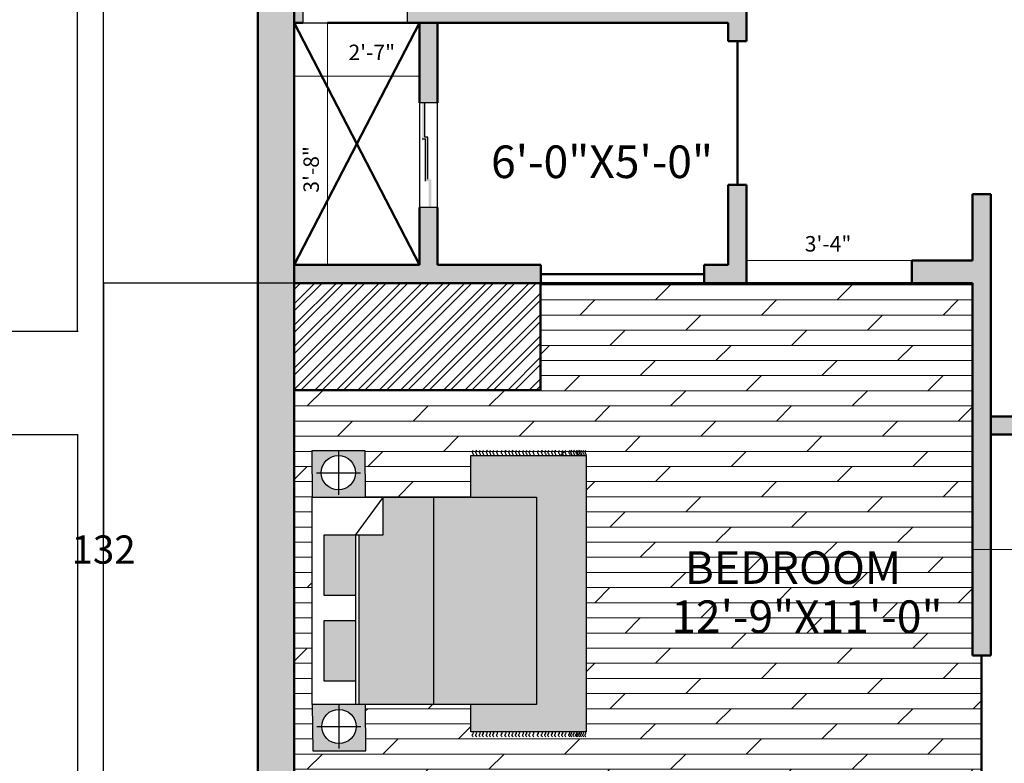
# Model space of a CAD drawing. Units: inches. Extents: x 1381 to 2246, y 1317 to 2168.
# Tile 11 of 15: x 1804 to 2048, y 1591 to 1776. Entities that reach past the tile are written whole.
import ezdxf

# ---------------------------------------------------------------- set-up
doc = ezdxf.new("R2010")
doc.units = ezdxf.units.IN
doc.header["$MEASUREMENT"] = 0
for name, color, linetype, lineweight in [('A-ANNO-DIMS', 2, 'Continuous', 18), ('A-ANNO-TEXT', 7, 'Continuous', 18), ('A-AREA-IDEN', 3, 'Continuous', 25), ('A-FLOR-PATT', 252, 'Continuous', 13), ('A-FURN', 8, 'Continuous', 18), ('A-GLAZ', 4, 'Continuous', 25), ('A-WALL', 7, 'Continuous', 50), ('A-WALL-PATT', 8, 'Continuous', 13)]:
    doc.layers.add(name, color=color, linetype=linetype, lineweight=lineweight)
doc.layers.add('furniture', color=250, linetype='Continuous')
doc.styles.get("Standard").update_dxf_attribs({"font": 'arial.ttf'})
doc.dimstyles.get("Standard").update_dxf_attribs({"dimtxt": 7, "dimasz": 0.18, "dimexe": 0.18, "dimexo": 0.0625, "dimgap": 0.09, "dimtad": 0, "dimtih": 1, "dimtoh": 1, "dimdec": 1, "dimzin": 0, "dimdsep": 46, "dimlunit": 3, "dimtxsty": 'Standard', "dimcen": 0.09, "dimadec": 0, "dimazin": 0, "dimtfac": 1, "dimtdec": 1, "dimtofl": 0, "dimtmove": 0, "dimatfit": 3, "dimfxl": 1, "dimtolj": 1, "dimtzin": 0, "dimarcsym": 0})

# ---------------------------------------------------------------- blocks, each defined once
blk = doc.blocks.new('CARPET')
at = {"layer": 'furniture'}
for p, q in [((-51.53, -98.11), (-51.53, -55.12)), ((-51.53, -55.12), (-41.27, -55.12)), ((36, -55.12), (51.55, -55.12)), ((51.55, -55.12), (51.55, -98.11)), ((51.55, -98.11), (-51.53, -98.11))]:
    blk.add_line(p, q, dxfattribs=at)
for points, knots in [([(-53.37, -55.99), (-53.22, -55.8), (-52.9, -55.41), (-52.34, -55.8), (-51.89, -56.08), (-51.65, -55.91), (-51.53, -55.83)], [0, 0, 0, 0, 0.653278, 1.290138, 1.740457, 2.114451, 2.114451, 2.114451, 2.114451]), ([(-53.37, -57.26), (-53.22, -57.07), (-52.9, -56.67), (-52.34, -57.07), (-51.89, -57.35), (-51.65, -57.17), (-51.53, -57.1)], [0, 0, 0, 0, 0.653278, 1.290138, 1.740457, 2.114451, 2.114451, 2.114451, 2.114451]), ([(-53.37, -58.59), (-53.22, -58.4), (-52.9, -58.01), (-52.34, -58.4), (-51.89, -58.68), (-51.65, -58.5), (-51.53, -58.43)], [0, 0, 0, 0, 0.653278, 1.290138, 1.740457, 2.114451, 2.114451, 2.114451, 2.114451]), ([(53.37, -55.99), (53.22, -55.8), (52.9, -55.41), (52.34, -55.8), (51.89, -56.08), (51.65, -55.91), (51.53, -55.83)], [0, 0, 0, 0, 0.653278, 1.290138, 1.740457, 2.114451, 2.114451, 2.114451, 2.114451]), ([(53.37, -57.26), (53.22, -57.07), (52.9, -56.67), (52.34, -57.07), (51.89, -57.35), (51.65, -57.17), (51.53, -57.1)], [0, 0, 0, 0, 0.653278, 1.290138, 1.740457, 2.114451, 2.114451, 2.114451, 2.114451]), ([(53.37, -58.59), (53.22, -58.4), (52.9, -58.01), (52.34, -58.4), (51.89, -58.68), (51.65, -58.5), (51.53, -58.43)], [0, 0, 0, 0, 0.653278, 1.290138, 1.740457, 2.114451, 2.114451, 2.114451, 2.114451]), ([(-53.37, -59.78), (-53.22, -59.58), (-52.9, -59.19), (-52.34, -59.58), (-51.89, -59.86), (-51.65, -59.69), (-51.53, -59.61)], [0, 0, 0, 0, 0.653278, 1.290138, 1.740457, 2.114451, 2.114451, 2.114451, 2.114451]), ([(-53.37, -61.22), (-53.22, -61.02), (-52.9, -60.63), (-52.34, -61.02), (-51.89, -61.3), (-51.65, -61.13), (-51.53, -61.05)], [0, 0, 0, 0, 0.653278, 1.290138, 1.740457, 2.114451, 2.114451, 2.114451, 2.114451]), ([(-53.37, -62.44), (-53.22, -62.25), (-52.9, -61.86), (-52.34, -62.25), (-51.89, -62.53), (-51.65, -62.36), (-51.53, -62.28)], [0, 0, 0, 0, 0.653278, 1.290138, 1.740457, 2.114451, 2.114451, 2.114451, 2.114451]), ([(53.37, -59.78), (53.22, -59.58), (52.9, -59.19), (52.34, -59.58), (51.89, -59.86), (51.65, -59.69), (51.53, -59.61)], [0, 0, 0, 0, 0.653278, 1.290138, 1.740457, 2.114451, 2.114451, 2.114451, 2.114451]), ([(53.37, -61.22), (53.22, -61.02), (52.9, -60.63), (52.34, -61.02), (51.89, -61.3), (51.65, -61.13), (51.53, -61.05)], [0, 0, 0, 0, 0.653278, 1.290138, 1.740457, 2.114451, 2.114451, 2.114451, 2.114451]), ([(53.37, -62.44), (53.22, -62.25), (52.9, -61.86), (52.34, -62.25), (51.89, -62.53), (51.65, -62.36), (51.53, -62.28)], [0, 0, 0, 0, 0.653278, 1.290138, 1.740457, 2.114451, 2.114451, 2.114451, 2.114451]), ([(-53.37, -63.63), (-53.22, -63.43), (-52.9, -63.04), (-52.34, -63.43), (-51.89, -63.72), (-51.65, -63.54), (-51.53, -63.46)], [0, 0, 0, 0, 0.653278, 1.290138, 1.740457, 2.114451, 2.114451, 2.114451, 2.114451]), ([(-53.37, -65.07), (-53.22, -64.87), (-52.9, -64.48), (-52.34, -64.87), (-51.89, -65.15), (-51.65, -64.98), (-51.53, -64.9)], [0, 0, 0, 0, 0.653278, 1.290138, 1.740457, 2.114451, 2.114451, 2.114451, 2.114451]), ([(53.37, -63.63), (53.22, -63.43), (52.9, -63.04), (52.34, -63.43), (51.89, -63.72), (51.65, -63.54), (51.53, -63.46)], [0, 0, 0, 0, 0.653278, 1.290138, 1.740457, 2.114451, 2.114451, 2.114451, 2.114451]), ([(53.37, -65.07), (53.22, -64.87), (52.9, -64.48), (52.34, -64.87), (51.89, -65.15), (51.65, -64.98), (51.53, -64.9)], [0, 0, 0, 0, 0.653278, 1.290138, 1.740457, 2.114451, 2.114451, 2.114451, 2.114451]), ([(-53.37, -66.76), (-53.22, -66.56), (-52.9, -66.17), (-52.34, -66.56), (-51.89, -66.84), (-51.65, -66.67), (-51.53, -66.59)], [0, 0, 0, 0, 0.653278, 1.290138, 1.740457, 2.114451, 2.114451, 2.114451, 2.114451]), ([(-53.37, -68.2), (-53.22, -68), (-52.9, -67.61), (-52.34, -68), (-51.89, -68.28), (-51.65, -68.11), (-51.53, -68.03)], [0, 0, 0, 0, 0.653278, 1.290138, 1.740457, 2.114451, 2.114451, 2.114451, 2.114451]), ([(-53.37, -69.53), (-53.22, -69.33), (-52.9, -68.94), (-52.34, -69.33), (-51.89, -69.61), (-51.65, -69.44), (-51.53, -69.36)], [0, 0, 0, 0, 0.653278, 1.290138, 1.740457, 2.114451, 2.114451, 2.114451, 2.114451]), ([(53.37, -66.76), (53.22, -66.56), (52.9, -66.17), (52.34, -66.56), (51.89, -66.84), (51.65, -66.67), (51.53, -66.59)], [0, 0, 0, 0, 0.653278, 1.290138, 1.740457, 2.114451, 2.114451, 2.114451, 2.114451]), ([(53.37, -68.2), (53.22, -68), (52.9, -67.61), (52.34, -68), (51.89, -68.28), (51.65, -68.11), (51.53, -68.03)], [0, 0, 0, 0, 0.653278, 1.290138, 1.740457, 2.114451, 2.114451, 2.114451, 2.114451]), ([(53.37, -69.53), (53.22, -69.33), (52.9, -68.94), (52.34, -69.33), (51.89, -69.61), (51.65, -69.44), (51.53, -69.36)], [0, 0, 0, 0, 0.653278, 1.290138, 1.740457, 2.114451, 2.114451, 2.114451, 2.114451]), ([(-53.37, -70.79), (-53.22, -70.6), (-52.9, -70.21), (-52.34, -70.6), (-51.89, -70.88), (-51.65, -70.7), (-51.53, -70.63)], [0, 0, 0, 0, 0.653278, 1.290138, 1.740457, 2.114451, 2.114451, 2.114451, 2.114451]), ([(-53.37, -72.12), (-53.22, -71.93), (-52.9, -71.54), (-52.34, -71.93), (-51.89, -72.21), (-51.65, -72.04), (-51.53, -71.96)], [0, 0, 0, 0, 0.653278, 1.290138, 1.740457, 2.114451, 2.114451, 2.114451, 2.114451]), ([(-53.37, -73.31), (-53.22, -73.11), (-52.9, -72.72), (-52.34, -73.11), (-51.89, -73.4), (-51.65, -73.22), (-51.53, -73.14)], [0, 0, 0, 0, 0.653278, 1.290138, 1.740457, 2.114451, 2.114451, 2.114451, 2.114451]), ([(53.37, -70.79), (53.22, -70.6), (52.9, -70.21), (52.34, -70.6), (51.89, -70.88), (51.65, -70.7), (51.53, -70.63)], [0, 0, 0, 0, 0.653278, 1.290138, 1.740457, 2.114451, 2.114451, 2.114451, 2.114451]), ([(53.37, -72.12), (53.22, -71.93), (52.9, -71.54), (52.34, -71.93), (51.89, -72.21), (51.65, -72.04), (51.53, -71.96)], [0, 0, 0, 0, 0.653278, 1.290138, 1.740457, 2.114451, 2.114451, 2.114451, 2.114451]), ([(53.37, -73.31), (53.22, -73.11), (52.9, -72.72), (52.34, -73.11), (51.89, -73.4), (51.65, -73.22), (51.53, -73.14)], [0, 0, 0, 0, 0.653278, 1.290138, 1.740457, 2.114451, 2.114451, 2.114451, 2.114451]), ([(-53.37, -74.75), (-53.22, -74.55), (-52.9, -74.16), (-52.34, -74.55), (-51.89, -74.83), (-51.65, -74.66), (-51.53, -74.58)], [0, 0, 0, 0, 0.653278, 1.290138, 1.740457, 2.114451, 2.114451, 2.114451, 2.114451]), ([(-53.37, -75.98), (-53.22, -75.78), (-52.9, -75.39), (-52.34, -75.78), (-51.89, -76.06), (-51.65, -75.89), (-51.53, -75.81)], [0, 0, 0, 0, 0.653278, 1.290138, 1.740457, 2.114451, 2.114451, 2.114451, 2.114451]), ([(-53.37, -77.16), (-53.22, -76.96), (-52.9, -76.57), (-52.34, -76.96), (-51.89, -77.25), (-51.65, -77.07), (-51.53, -76.99)], [0, 0, 0, 0, 0.653278, 1.290138, 1.740457, 2.114451, 2.114451, 2.114451, 2.114451]), ([(53.37, -74.75), (53.22, -74.55), (52.9, -74.16), (52.34, -74.55), (51.89, -74.83), (51.65, -74.66), (51.53, -74.58)], [0, 0, 0, 0, 0.653278, 1.290138, 1.740457, 2.114451, 2.114451, 2.114451, 2.114451]), ([(53.37, -75.98), (53.22, -75.78), (52.9, -75.39), (52.34, -75.78), (51.89, -76.06), (51.65, -75.89), (51.53, -75.81)], [0, 0, 0, 0, 0.653278, 1.290138, 1.740457, 2.114451, 2.114451, 2.114451, 2.114451]), ([(53.37, -77.16), (53.22, -76.96), (52.9, -76.57), (52.34, -76.96), (51.89, -77.25), (51.65, -77.07), (51.53, -76.99)], [0, 0, 0, 0, 0.653278, 1.290138, 1.740457, 2.114451, 2.114451, 2.114451, 2.114451]), ([(-53.37, -78.6), (-53.22, -78.4), (-52.9, -78.01), (-52.34, -78.4), (-51.89, -78.68), (-51.65, -78.51), (-51.53, -78.43)], [0, 0, 0, 0, 0.653278, 1.290138, 1.740457, 2.114451, 2.114451, 2.114451, 2.114451]), ([(-53.37, -80.29), (-53.22, -80.09), (-52.9, -79.7), (-52.34, -80.09), (-51.89, -80.37), (-51.65, -80.2), (-51.53, -80.12)], [0, 0, 0, 0, 0.653278, 1.290138, 1.740457, 2.114451, 2.114451, 2.114451, 2.114451]), ([(53.37, -78.6), (53.22, -78.4), (52.9, -78.01), (52.34, -78.4), (51.89, -78.68), (51.65, -78.51), (51.53, -78.43)], [0, 0, 0, 0, 0.653278, 1.290138, 1.740457, 2.114451, 2.114451, 2.114451, 2.114451]), ([(53.37, -80.29), (53.22, -80.09), (52.9, -79.7), (52.34, -80.09), (51.89, -80.37), (51.65, -80.2), (51.53, -80.12)], [0, 0, 0, 0, 0.653278, 1.290138, 1.740457, 2.114451, 2.114451, 2.114451, 2.114451]), ([(-53.37, -81.73), (-53.22, -81.53), (-52.9, -81.14), (-52.34, -81.53), (-51.89, -81.81), (-51.65, -81.64), (-51.53, -81.56)], [0, 0, 0, 0, 0.653278, 1.290138, 1.740457, 2.114451, 2.114451, 2.114451, 2.114451]), ([(-53.37, -83.06), (-53.22, -82.86), (-52.9, -82.47), (-52.34, -82.86), (-51.89, -83.14), (-51.65, -82.97), (-51.53, -82.89)], [0, 0, 0, 0, 0.653278, 1.290138, 1.740457, 2.114451, 2.114451, 2.114451, 2.114451]), ([(-53.37, -84.18), (-53.22, -83.99), (-52.9, -83.6), (-52.34, -83.99), (-51.89, -84.27), (-51.65, -84.09), (-51.53, -84.02)], [0, 0, 0, 0, 0.653278, 1.290138, 1.740457, 2.114451, 2.114451, 2.114451, 2.114451]), ([(53.37, -81.73), (53.22, -81.53), (52.9, -81.14), (52.34, -81.53), (51.89, -81.81), (51.65, -81.64), (51.53, -81.56)], [0, 0, 0, 0, 0.653278, 1.290138, 1.740457, 2.114451, 2.114451, 2.114451, 2.114451]), ([(53.37, -83.06), (53.22, -82.86), (52.9, -82.47), (52.34, -82.86), (51.89, -83.14), (51.65, -82.97), (51.53, -82.89)], [0, 0, 0, 0, 0.653278, 1.290138, 1.740457, 2.114451, 2.114451, 2.114451, 2.114451]), ([(53.37, -84.18), (53.22, -83.99), (52.9, -83.6), (52.34, -83.99), (51.89, -84.27), (51.65, -84.09), (51.53, -84.02)], [0, 0, 0, 0, 0.653278, 1.290138, 1.740457, 2.114451, 2.114451, 2.114451, 2.114451]), ([(-53.37, -85.51), (-53.22, -85.32), (-52.9, -84.93), (-52.34, -85.32), (-51.89, -85.6), (-51.65, -85.42), (-51.53, -85.35)], [0, 0, 0, 0, 0.653278, 1.290138, 1.740457, 2.114451, 2.114451, 2.114451, 2.114451]), ([(-53.37, -86.7), (-53.22, -86.5), (-52.9, -86.11), (-52.34, -86.5), (-51.89, -86.78), (-51.65, -86.61), (-51.53, -86.53)], [0, 0, 0, 0, 0.653278, 1.290138, 1.740457, 2.114451, 2.114451, 2.114451, 2.114451]), ([(-53.37, -88.14), (-53.22, -87.94), (-52.9, -87.55), (-52.34, -87.94), (-51.89, -88.22), (-51.65, -88.05), (-51.53, -87.97)], [0, 0, 0, 0, 0.653278, 1.290138, 1.740457, 2.114451, 2.114451, 2.114451, 2.114451]), ([(53.37, -85.51), (53.22, -85.32), (52.9, -84.93), (52.34, -85.32), (51.89, -85.6), (51.65, -85.42), (51.53, -85.35)], [0, 0, 0, 0, 0.653278, 1.290138, 1.740457, 2.114451, 2.114451, 2.114451, 2.114451]), ([(53.37, -86.7), (53.22, -86.5), (52.9, -86.11), (52.34, -86.5), (51.89, -86.78), (51.65, -86.61), (51.53, -86.53)], [0, 0, 0, 0, 0.653278, 1.290138, 1.740457, 2.114451, 2.114451, 2.114451, 2.114451]), ([(53.37, -88.14), (53.22, -87.94), (52.9, -87.55), (52.34, -87.94), (51.89, -88.22), (51.65, -88.05), (51.53, -87.97)], [0, 0, 0, 0, 0.653278, 1.290138, 1.740457, 2.114451, 2.114451, 2.114451, 2.114451]), ([(-53.37, -89.36), (-53.22, -89.17), (-52.9, -88.78), (-52.34, -89.17), (-51.89, -89.45), (-51.65, -89.28), (-51.53, -89.2)], [0, 0, 0, 0, 0.653278, 1.290138, 1.740457, 2.114451, 2.114451, 2.114451, 2.114451]), ([(-53.37, -90.55), (-53.22, -90.35), (-52.9, -89.96), (-52.34, -90.35), (-51.89, -90.64), (-51.65, -90.46), (-51.53, -90.38)], [0, 0, 0, 0, 0.653278, 1.290138, 1.740457, 2.114451, 2.114451, 2.114451, 2.114451]), ([(-53.37, -91.99), (-53.22, -91.79), (-52.9, -91.4), (-52.34, -91.79), (-51.89, -92.07), (-51.65, -91.9), (-51.53, -91.82)], [0, 0, 0, 0, 0.653278, 1.290138, 1.740457, 2.114451, 2.114451, 2.114451, 2.114451]), ([(53.37, -89.36), (53.22, -89.17), (52.9, -88.78), (52.34, -89.17), (51.89, -89.45), (51.65, -89.28), (51.53, -89.2)], [0, 0, 0, 0, 0.653278, 1.290138, 1.740457, 2.114451, 2.114451, 2.114451, 2.114451]), ([(53.37, -90.55), (53.22, -90.35), (52.9, -89.96), (52.34, -90.35), (51.9, -90.63), (51.66, -90.47), (51.55, -90.4)], [0, 0, 0, 0, 0.653278, 1.290138, 1.740457, 2.0926, 2.0926, 2.0926, 2.0926]), ([(53.37, -91.99), (53.22, -91.79), (52.9, -91.4), (52.34, -91.79), (51.9, -92.07), (51.66, -91.91), (51.55, -91.83)], [0, 0, 0, 0, 0.653278, 1.290138, 1.740457, 2.0926, 2.0926, 2.0926, 2.0926]), ([(-53.37, -92.69), (-53.22, -92.48), (-52.9, -92.08), (-52.35, -92.49), (-51.89, -92.77), (-51.65, -92.6), (-51.53, -92.52)], [0, 0, 0, 0, 0.663904, 1.307406, 1.757725, 2.131719, 2.131719, 2.131719, 2.131719]), ([(-53.37, -93.61), (-53.22, -93.42), (-52.9, -93.03), (-52.34, -93.42), (-51.89, -93.7), (-51.65, -93.52), (-51.53, -93.45)], [0, 0, 0, 0, 0.653278, 1.290138, 1.740457, 2.114451, 2.114451, 2.114451, 2.114451]), ([(-53.37, -94.55), (-53.22, -94.35), (-52.9, -93.96), (-52.34, -94.35), (-51.89, -94.63), (-51.65, -94.46), (-51.53, -94.38)], [0, 0, 0, 0, 0.653278, 1.290138, 1.740457, 2.114451, 2.114451, 2.114451, 2.114451]), ([(-53.37, -95.05), (-53.22, -94.85), (-52.9, -94.46), (-52.34, -94.85), (-51.89, -95.14), (-51.65, -94.96), (-51.53, -94.88)], [0, 0, 0, 0, 0.653278, 1.290138, 1.740457, 2.114451, 2.114451, 2.114451, 2.114451]), ([(-53.37, -95.73), (-53.22, -95.54), (-52.9, -95.15), (-52.34, -95.54), (-51.89, -95.82), (-51.65, -95.65), (-51.53, -95.57)], [0, 0, 0, 0, 0.653278, 1.290138, 1.740457, 2.114451, 2.114451, 2.114451, 2.114451]), ([(53.37, -95.78), (53.22, -95.58), (52.9, -95.19), (52.34, -95.58), (51.89, -95.86), (51.65, -95.69), (51.53, -95.61)], [0, 0, 0, 0, 0.653278, 1.290138, 1.740457, 2.114451, 2.114451, 2.114451, 2.114451]), ([(53.37, -92.69), (53.22, -92.49), (52.9, -92.09), (52.34, -92.49), (51.9, -92.77), (51.66, -92.61), (51.55, -92.53)], [0, 0, 0, 0, 0.656792, 1.295826, 1.746145, 2.098292, 2.098292, 2.098292, 2.098292]), ([(53.37, -93.66), (53.22, -93.46), (52.9, -93.07), (52.34, -93.46), (51.9, -93.74), (51.66, -93.58), (51.55, -93.5)], [0, 0, 0, 0, 0.653278, 1.290138, 1.740457, 2.0926, 2.0926, 2.0926, 2.0926]), ([(53.37, -94.59), (53.22, -94.4), (52.9, -94.01), (52.34, -94.4), (51.9, -94.68), (51.66, -94.51), (51.55, -94.44)], [0, 0, 0, 0, 0.653278, 1.290138, 1.740457, 2.0926, 2.0926, 2.0926, 2.0926]), ([(53.37, -95.1), (53.22, -94.9), (52.9, -94.51), (52.34, -94.9), (51.9, -95.18), (51.66, -95.02), (51.55, -94.94)], [0, 0, 0, 0, 0.653278, 1.290138, 1.740457, 2.0926, 2.0926, 2.0926, 2.0926]), ([(-53.37, -96.38), (-53.22, -96.18), (-52.9, -95.79), (-52.34, -96.18), (-51.89, -96.47), (-51.65, -96.29), (-51.53, -96.21)], [0, 0, 0, 0, 0.653278, 1.290138, 1.740457, 2.114451, 2.114451, 2.114451, 2.114451]), ([(-53.37, -97.17), (-53.22, -96.98), (-52.9, -96.59), (-52.34, -96.98), (-51.89, -97.26), (-51.65, -97.08), (-51.53, -97.01)], [0, 0, 0, 0, 0.653278, 1.290138, 1.740457, 2.114451, 2.114451, 2.114451, 2.114451]), ([(-53.37, -97.99), (-53.22, -97.79), (-52.9, -97.4), (-52.34, -97.79), (-51.89, -98.08), (-51.65, -97.9), (-51.53, -97.82)], [0, 0, 0, 0, 0.653278, 1.290138, 1.740457, 2.114451, 2.114451, 2.114451, 2.114451]), ([(53.37, -96.43), (53.22, -96.23), (52.9, -95.84), (52.34, -96.23), (51.89, -96.51), (51.65, -96.34), (51.53, -96.26)], [0, 0, 0, 0, 0.653278, 1.290138, 1.740457, 2.114451, 2.114451, 2.114451, 2.114451]), ([(53.37, -97.22), (53.22, -97.02), (52.9, -96.63), (52.34, -97.02), (51.89, -97.3), (51.65, -97.13), (51.53, -97.05)], [0, 0, 0, 0, 0.653278, 1.290138, 1.740457, 2.114451, 2.114451, 2.114451, 2.114451]), ([(53.37, -97.99), (53.22, -97.79), (52.9, -97.4), (52.34, -97.79), (51.89, -98.08), (51.65, -97.9), (51.53, -97.82)], [0, 0, 0, 0, 0.653278, 1.290138, 1.740457, 2.114451, 2.114451, 2.114451, 2.114451])]:
    blk.add_open_spline(points, degree=3, knots=knots, dxfattribs=at)
blk = doc.blocks.new('A$C58D270C6')
at = {"layer": 'furniture'}
for p, q in [((9.09, 124.13), (9.09, 108.87)), ((1.46, 116.5), (16.73, 116.5)), ((14.97, 94.84), (24.62, 107.92)), ((24.62, 94.93), (24.62, 107.92)), ((42.08, 108), (42.08, 36)), ((14.97, 94.93), (24.62, 94.93)), ((14.97, 94.84), (14.97, 36)), ((16.22, 94.93), (16.22, 36)), ((9.25, 36), (9.25, 20.74)), ((1.62, 28.37), (16.88, 28.37))]:
    blk.add_line(p, q, dxfattribs=at)
for points in [[(18.5, 108), (18.34, 124.13), (-0.16, 124.13), (0, 108)], [(0, 108), (77.91, 108), (77.91, 36), (0, 36)], [(4.09, 94.93), (14.97, 94.93), (14.97, 73.83), (4.09, 73.83)], [(4.09, 65.23), (14.97, 65.23), (14.97, 44.13), (4.09, 44.13)], [(18.65, 19.87), (18.5, 36), (0, 36), (0.16, 19.87)]]:
    blk.add_lwpolyline(points, close=True, dxfattribs=at)
for centre in [(9.09, 116.5), (9.25, 28.37)]:
    blk.add_circle(centre, 5.95, dxfattribs=at)
at = {"layer": 'furniture', "xscale": 0.9312884925094044, "yscale": 0.9312884925094044, "zscale": 0.9312884925094044, "rotation": 90}
blk.add_blockref('CARPET', (3.79, 74.47), dxfattribs=at)
blk = doc.blocks.new('*D60')
at = {"layer": 'A-ANNO-DIMS', "color": 0, "lineweight": -2, "transparency": 16777216}
for p, q in [((1737.61, 1672.92), (1818.27, 1672.92)), ((1818.09, 1672.74), (1818.09, 1576.08)), ((1818.09, 1472.1), (1818.09, 1568.75)), ((1737.61, 1471.92), (1818.27, 1471.92))]:
    blk.add_line(p, q, dxfattribs=at)
at = {"layer": 'A-ANNO-DIMS', "color": 0, "transparency": 16777216}
for points in [[(1818.06, 1672.74), (1818.12, 1672.74), (1818.09, 1672.92)], [(1818.06, 1472.1), (1818.12, 1472.1), (1818.09, 1471.92)]]:
    blk.add_solid(points, dxfattribs=at)
at = {"layer": 'Defpoints', "color": 0, "transparency": 16777216}
for p in [(1737.55, 1672.92), (1818.09, 1672.92), (1737.55, 1471.92)]:
    blk.add_point(p, dxfattribs=at)
at = {"layer": 'A-ANNO-DIMS', "color": 0, "transparency": 16777216, "insert": (1818.09, 1572.42), "char_height": 7, "attachment_point": 5}
blk.add_mtext('\\A1;201', dxfattribs=at)
blk = doc.blocks.new('*D61')
at = {"layer": 'A-ANNO-DIMS', "color": 0, "lineweight": -2, "transparency": 16777216}
for p, q in [((1737.61, 1911.42), (1818.27, 1911.42)), ((1818.09, 1911.24), (1818.09, 1808.63)), ((1818.09, 1698.7), (1818.09, 1801.3)), ((1737.61, 1698.52), (1818.27, 1698.52))]:
    blk.add_line(p, q, dxfattribs=at)
at = {"layer": 'A-ANNO-DIMS', "color": 0, "transparency": 16777216}
for points in [[(1818.06, 1911.24), (1818.12, 1911.24), (1818.09, 1911.42)], [(1818.06, 1698.7), (1818.12, 1698.7), (1818.09, 1698.52)]]:
    blk.add_solid(points, dxfattribs=at)
at = {"layer": 'Defpoints', "color": 0, "transparency": 16777216}
for p in [(1737.55, 1911.42), (1818.09, 1911.42), (1737.55, 1698.52)]:
    blk.add_point(p, dxfattribs=at)
at = {"layer": 'A-ANNO-DIMS', "color": 0, "transparency": 16777216, "insert": (1818.09, 1804.97), "char_height": 7, "attachment_point": 5}
blk.add_mtext('\\A1;212.9', dxfattribs=at)
blk = doc.blocks.new('*D76')
at = {"layer": 'A-ANNO-DIMS', "color": 0, "lineweight": -2, "transparency": 16777216}
for p, q in [((1862.74, 2092.92), (1824.38, 2092.92)), ((1824.56, 2092.74), (1824.56, 1786.08)), ((1824.56, 1472.1), (1824.56, 1778.75)), ((1862.74, 1471.92), (1824.38, 1471.92))]:
    blk.add_line(p, q, dxfattribs=at)
at = {"layer": 'A-ANNO-DIMS', "color": 0, "transparency": 16777216}
for points in [[(1824.53, 2092.74), (1824.59, 2092.74), (1824.56, 2092.92)], [(1824.53, 1472.1), (1824.59, 1472.1), (1824.56, 1471.92)]]:
    blk.add_solid(points, dxfattribs=at)
at = {"layer": 'Defpoints', "color": 0, "transparency": 16777216}
for p in [(1824.56, 2092.92), (1862.81, 2092.92), (1862.81, 1471.92)]:
    blk.add_point(p, dxfattribs=at)
at = {"layer": 'A-ANNO-DIMS', "color": 0, "transparency": 16777216, "insert": (1824.56, 1782.42), "char_height": 7, "attachment_point": 5}
blk.add_mtext('\\A1;621', dxfattribs=at)
blk = doc.blocks.new('*D81')
at = {"layer": 'A-ANNO-DIMS', "color": 0, "lineweight": -2, "transparency": 16777216}
for p, q in [((1871.74, 1710.42), (1824.38, 1710.42)), ((1824.56, 1710.24), (1824.56, 1648.08)), ((1824.56, 1578.6), (1824.56, 1640.75)), ((1871.74, 1578.42), (1824.38, 1578.42))]:
    blk.add_line(p, q, dxfattribs=at)
at = {"layer": 'A-ANNO-DIMS', "color": 0, "transparency": 16777216}
for points in [[(1824.53, 1710.24), (1824.59, 1710.24), (1824.56, 1710.42)], [(1824.53, 1578.6), (1824.59, 1578.6), (1824.56, 1578.42)]]:
    blk.add_solid(points, dxfattribs=at)
at = {"layer": 'Defpoints', "color": 0, "transparency": 16777216}
for p in [(1824.56, 1710.42), (1871.81, 1710.42), (1871.81, 1578.42)]:
    blk.add_point(p, dxfattribs=at)
at = {"layer": 'A-ANNO-DIMS', "color": 0, "transparency": 16777216, "insert": (1824.56, 1644.42), "char_height": 7, "attachment_point": 5}
blk.add_mtext('\\A1;132', dxfattribs=at)

msp = doc.modelspace()

# ---------------------------------------------------------------- hatches: boundary and pattern name
at = {"layer": 'A-FLOR-PATT'}
h = msp.add_hatch(dxfattribs=at)
h.set_pattern_fill('ANSI32', color=256, scale=10)
h.set_pattern_definition([(45, (415.7542, 0), (-2.6516504, 2.6516504), []), (45, (417.522, 0), (-2.6516504, 2.6516504), [])])
h.paths.add_polyline_path([(1932.8736, 1710.4163), (1871.8052, 1710.4163), (1871.8052, 1683.9148), (1932.8736, 1683.9148)])
h = msp.add_hatch(dxfattribs=at)
h.set_pattern_fill('DOLMIT', color=256, scale=15)
h.paths.add_polyline_path([(2039.8052, 1710.4163), (2024.8052, 1710.4163), (1932.7523, 1710.4163), (1932.7523, 1683.9148), (1871.8052, 1683.9148), (1871.8052, 1578.4163), (2039.8052, 1578.4163), (2039.8052, 1581.7679), (2042.0552, 1581.7679), (2042.0552, 1618.2205), (2039.8052, 1618.2205)])
edge = h.paths.add_edge_path(flags=16)
edge.add_spline(control_points=[(1941.6512, 1599.2474), (1941.7034, 1599.1739), (1941.8185, 1599.0119), (1941.6311, 1598.7103), (1941.372, 1598.3387), (1941.6312, 1598.1308), (1941.7624, 1598.0254)], knot_values=[0, 0, 0, 0, 0.37399428, 0.82431366, 1.46117297, 2.11445126, 2.11445126, 2.11445126, 2.11445126], degree=3, periodic=0)
edge.add_spline(control_points=[(1941.9859, 1599.2474), (1942.0381, 1599.1739), (1942.1532, 1599.0119), (1941.9659, 1598.7103), (1941.7067, 1598.3387), (1941.9659, 1598.1308), (1942.0971, 1598.0254)], knot_values=[0, 0, 0, 0, 0.37399428, 0.82431366, 1.46117297, 2.11445126, 2.11445126, 2.11445126, 2.11445126], degree=3, periodic=0)
edge = h.paths.add_edge_path(flags=16)
edge.add_line((1944.1282, 1667.7293), (1944.1282, 1599.2474))
edge.add_line((1944.1282, 1599.2474), (1915.5728, 1599.2474))
edge.add_line((1915.5728, 1599.2474), (1915.5728, 1606.0382))
edge.add_line((1915.5728, 1606.0382), (1889.4451, 1606.0382))
edge.add_line((1889.4451, 1606.0382), (1889.5561, 1594.5315))
edge.add_line((1889.5561, 1594.5315), (1876.3603, 1594.5315))
edge.add_line((1876.3603, 1594.5315), (1876.2493, 1606.0382))
edge.add_line((1876.2493, 1606.0382), (1876.2493, 1657.3975))
edge.add_line((1876.2493, 1657.3975), (1876.1383, 1668.9042))
edge.add_line((1876.1383, 1668.9042), (1889.3342, 1668.9042))
edge.add_line((1889.3342, 1668.9042), (1889.4451, 1657.3975))
edge.add_line((1889.4451, 1657.3975), (1915.5728, 1657.3975))
edge.add_line((1915.5728, 1657.3975), (1915.5728, 1667.7293))
edge.add_line((1915.5728, 1667.7293), (1941.69, 1667.7293))
edge.add_spline(control_points=[(1941.69, 1667.7293), (1941.7379, 1667.7989), (1941.8471, 1667.9576), (1941.661, 1668.2542), (1941.4024, 1668.626), (1941.6615, 1668.8339), (1941.7927, 1668.9392)], knot_values=[0, 0, 0, 0, 0.3521435, 0.80246288, 1.43932219, 2.09260048, 2.09260048, 2.09260048, 2.09260048], degree=3, periodic=0)
edge.add_spline(control_points=[(1942.1275, 1668.9392), (1941.9963, 1668.8339), (1941.7372, 1668.626), (1941.9957, 1668.2542), (1942.1818, 1667.9576), (1942.0727, 1667.7989), (1942.0248, 1667.7293)], knot_values=[0, 0, 0, 0, 0.65327829, 1.2901376, 1.74045698, 2.09260048, 2.09260048, 2.09260048, 2.09260048], degree=3, periodic=0)
edge.add_line((1942.0248, 1667.7293), (1944.1282, 1667.7293))
h.paths.add_polyline_path([(1893.809, 1657.3422), (1893.809, 1648.0757), (1886.9767, 1648.0757), (1886.9307, 1648.0133), (1886.9307, 1611.8376), (1879.1699, 1611.8376), (1879.1699, 1626.8866), (1886.9307, 1626.8866), (1886.9307, 1633.0267), (1879.1699, 1633.0267), (1879.1699, 1648.0757), (1886.9767, 1648.0757)], flags=0)
h.paths.add_polyline_path([(1886.984, 1663.4608, -1), (1878.4885, 1663.4608, -1)], flags=0)
h.paths.add_polyline_path([(1887.0949, 1600.5947, -1), (1878.5995, 1600.5947, -1)], flags=0)
h.paths.add_polyline_path([(1963.1209, 1621.5603), (2032.2362, 1621.5603), (2032.2362, 1633.9282), (1963.1209, 1633.9282)], flags=24)
h.paths.add_polyline_path([(1966.4202, 1633.6986), (2028.882, 1633.6986), (2028.882, 1646.2317), (1966.4202, 1646.2317)], flags=24)
at = {"layer": 'A-FURN'}
h = msp.add_hatch(color=256, dxfattribs=at)
h.dxf.hatch_style = 1
h.paths.add_polyline_path([(1944.1282, 1667.7293), (1915.5728, 1667.7293), (1915.5728, 1657.3975), (1931.8208, 1657.3975), (1931.8208, 1606.0382), (1915.5728, 1606.0382), (1915.5728, 1599.2474), (1944.1282, 1599.2474)])
h.paths.add_polyline_path([(1882.8472, 1606.0382), (1876.2493, 1606.0382), (1876.3603, 1594.5315), (1889.5561, 1594.5315), (1889.4451, 1606.0382), (1882.8472, 1606.0382), (1882.8472, 1604.8424, -0.41421356), (1887.0949, 1600.5947, -1), (1878.5995, 1600.5947, -0.41421356), (1882.8472, 1604.8424)])
h.paths.add_polyline_path([(1889.3342, 1668.9042), (1882.7362, 1668.9042), (1882.7362, 1667.7085, -0.41421356), (1886.984, 1663.4608, -1), (1878.4885, 1663.4608, -0.41421356), (1882.7362, 1667.7085), (1882.7362, 1668.9042), (1876.1383, 1668.9042), (1876.2493, 1657.3975), (1889.4451, 1657.3975)])
h = msp.add_hatch(color=256, dxfattribs=at)
h.dxf.hatch_style = 1
h.paths.add_polyline_path([(1906.2646, 1657.3975), (1893.8498, 1657.3975), (1893.809, 1657.3422), (1893.809, 1648.0757), (1887.8171, 1648.0757), (1887.8171, 1606.0382), (1906.2646, 1606.0382)])
h.paths.add_polyline_path([(1931.8208, 1657.3975), (1906.2646, 1657.3975), (1906.2646, 1606.0382), (1931.8208, 1606.0382)])
h = msp.add_hatch(color=256, dxfattribs=at)
h.dxf.hatch_style = 1
h.paths.add_polyline_path([(1886.9307, 1626.8866), (1879.1699, 1626.8866), (1879.1699, 1611.8376), (1886.9307, 1611.8376)])
h.paths.add_polyline_path([(1886.9307, 1648.0757), (1879.1699, 1648.0757), (1879.1699, 1633.0267), (1886.9307, 1633.0267)])
at = {"layer": 'A-GLAZ'}
h = msp.add_hatch(color=256, dxfattribs=at)
h.dxf.hatch_style = 1
h.paths.add_polyline_path([(1904.8793, 1736.1591), (1904.8793, 1746.5538), (1904.1533, 1746.5538), (1904.1533, 1755.1129), (1903.4932, 1755.1129), (1903.4932, 1746.1133), (1904.2633, 1746.1133), (1904.2633, 1735.6746), (1905.0552, 1735.6746), (1905.0552, 1729.193), (1905.7814, 1729.193), (1905.7814, 1736.1591)])
at = {"layer": 'A-WALL-PATT'}
h = msp.add_hatch(color=256, dxfattribs=at)
h.dxf.hatch_style = 1
h.paths.add_polyline_path([(1990.4785, 1915.9163), (1929.807, 1915.9163), (1929.807, 1911.4163), (1990.4785, 1911.4163)], flags=17)
h.paths.add_polyline_path([(1900.7902, 1915.9163), (1871.8052, 1915.9163), (1871.8052, 1911.4163), (1900.7902, 1911.4163)], flags=17)
h.paths.add_polyline_path([(2043.2216, 1915.9163), (2038.3052, 1915.9163), (2038.3052, 2035.4163), (2098.0373, 2035.4163), (2098.0373, 2039.9163), (2033.8052, 2039.9163), (2033.8052, 1915.9163), (2028.7731, 1915.9163), (2028.7731, 1911.4163), (2043.2216, 1911.4163)], flags=17)
h.paths.add_polyline_path([(2153.3052, 1915.9163), (2085.2216, 1915.9163), (2085.2216, 1911.4163), (2153.3052, 1911.4163)], flags=17)
h.paths.add_polyline_path([(1935.508, 1911.4163), (1931.008, 1911.4163), (1931.008, 1779.4163), (1899.8394, 1779.4163), (1899.8394, 1774.9163), (1902.8052, 1774.9163), (1979.3052, 1774.9163), (1979.3052, 1770.3401), (1983.8052, 1770.3401), (1983.8052, 1779.4163), (1935.508, 1779.4163)], flags=17)
h.paths.add_polyline_path([(1871.8052, 2083.9163), (2153.3052, 2083.9163), (2153.3052, 2039.9163), (2141.7178, 2039.9163), (2141.7178, 2035.4163), (2153.3052, 2035.4163), (2153.3052, 1471.9163), (2162.3052, 1471.9163), (2162.3052, 2092.9163), (1862.8052, 2092.9163), (1862.8052, 1471.9163), (1904.4174, 1471.9163), (1904.4174, 1480.9163), (1871.8052, 1480.9163), (1871.8052, 1569.4163), (1964.2348, 1569.4163), (1964.2348, 1578.4163), (1871.8052, 1578.4163)])
h.paths.add_polyline_path([(1907.3052, 1729.193), (1902.8052, 1729.193), (1902.8052, 1714.9163), (1871.8052, 1714.9163), (1871.8052, 1710.4163), (1932.8736, 1710.4163), (1932.8736, 1714.9163), (1907.3052, 1714.9163)], flags=17)
h.paths.add_polyline_path([(2044.3052, 1644.4163), (2039.8052, 1644.4163), (2039.8052, 1618.2205), (2044.3052, 1618.2205)], flags=17)
h.paths.add_polyline_path([(2044.3052, 1581.7679), (2039.8052, 1581.7679), (2039.8052, 1578.4163), (2027.577, 1578.4163), (2027.577, 1569.4163), (2044.3052, 1569.4163)], flags=17)
h = msp.add_hatch(color=256, dxfattribs=at)
h.dxf.hatch_style = 1
h.paths.add_polyline_path([(1873.9195, 1779.4163), (1871.8052, 1779.4163), (1871.8052, 1774.9163), (1873.9195, 1774.9163)])
h.paths.add_polyline_path([(1983.8052, 1779.4163), (1935.508, 1779.4163), (1935.508, 1911.4163), (1931.008, 1911.4163), (1931.008, 1779.4163), (1899.8394, 1779.4163), (1899.8394, 1774.9163), (1902.8052, 1774.9163), (1979.3052, 1774.9163), (1979.3052, 1770.3401), (1983.8052, 1770.3401)])
h.paths.add_polyline_path([(1907.3052, 1774.9163), (1902.8052, 1774.9163), (1902.8052, 1755.1129), (1907.3052, 1755.1129)])
h.paths.add_polyline_path([(1983.8052, 1734.7997), (1979.3052, 1734.7997), (1979.3052, 1714.9163), (1973.3503, 1714.9163), (1973.3503, 1710.4163), (1983.8052, 1710.4163)])
h.paths.add_polyline_path([(2044.3052, 1732.454), (2039.8052, 1732.454), (2039.8052, 1716.0149), (2024.8052, 1716.0149), (2024.8052, 1710.4163), (2039.8052, 1710.4163), (2039.8052, 1644.4163), (2044.3052, 1644.4163)])
h.paths.add_polyline_path([(2056.2659, 1677.4163), (2044.3052, 1677.4163), (2044.3052, 1672.9163), (2056.2659, 1672.9163)])
h.paths.add_polyline_path([(2119.6192, 1677.4163), (2104.2659, 1677.4163), (2104.2659, 1672.9163), (2119.6192, 1672.9163)])
h.paths.add_polyline_path([(2012.5552, 1480.9163), (1952.401, 1480.9163), (1952.401, 1471.9163), (2012.5552, 1471.9163)])
h.paths.add_polyline_path([(1870.8149, 1834.6368), (1933.6567, 1834.6368), (1933.6567, 1847.0047), (1870.8149, 1847.0047)], flags=9)

# ---------------------------------------------------------------- linework, layer by layer
at = {"layer": 'A-ANNO-DIMS'}
for p, q in [((1880.034, 1714.9163), (1880.034, 1774.9163)), ((1871.8052, 1761.653), (1902.8052, 1761.653)), ((1983.8052, 1716.0149), (2024.8052, 1716.0149)), ((2039.8052, 1644.4163), (2153.3052, 1644.4163))]:
    msp.add_line(p, q, dxfattribs=at)
at = {"layer": 'A-GLAZ'}
for p, q in [((1873.9195, 1779.4163), (1873.9195, 1774.9163)), ((1899.8394, 1774.9163), (1899.8394, 1779.4163)), ((1873.9195, 1774.9163), (1902.8052, 1774.9163)), ((1907.3052, 1755.1129), (1902.8052, 1755.1129)), ((1902.8052, 1755.1129), (1902.8052, 1729.193)), ((1904.1533, 1746.5538), (1904.1533, 1755.1129)), ((1907.3052, 1729.193), (1907.3052, 1755.1129)), ((1904.8793, 1746.5538), (1904.1533, 1746.5538)), ((1904.8793, 1736.1591), (1904.8793, 1746.5538)), ((1904.2633, 1746.1133), (1903.4932, 1746.1133)), ((1904.2633, 1735.6746), (1904.2633, 1746.1133)), ((1907.3052, 1729.193), (1902.8052, 1729.193))]:
    msp.add_line(p, q, dxfattribs=at)
at = {"layer": 'A-WALL'}
for p, q in [((1862.8052, 2092.9163), (1862.8052, 1471.9163)), ((1871.8052, 2083.9163), (1871.8052, 1578.4163)), ((1983.8052, 1779.4163), (1983.8052, 1770.3401)), ((1902.8052, 1714.9163), (1871.8052, 1774.9163)), ((1871.8052, 1714.9163), (1902.8052, 1774.9163)), ((1871.8052, 1774.9163), (1873.9195, 1774.9163)), ((1880.034, 1774.9163), (1979.3052, 1774.9163)), ((1902.8052, 1774.9163), (1902.8052, 1755.1129)), ((1907.3052, 1774.9163), (1907.3052, 1755.1129)), ((1979.3052, 1774.9163), (1979.3052, 1770.3401)), ((1979.3052, 1770.3401), (1983.8052, 1770.3401)), ((1981.5552, 1734.7997), (1981.5552, 1770.3401)), ((1979.3052, 1734.7997), (1979.3052, 1714.9163)), ((1979.3052, 1734.7997), (1983.8052, 1734.7997)), ((1983.8052, 1734.7997), (1983.8052, 1710.4163)), ((2039.8052, 1732.454), (2044.3052, 1732.454)), ((2039.8052, 1732.454), (2039.8052, 1716.0149)), ((2044.3052, 1732.454), (2044.3052, 1618.2205)), ((1902.8052, 1729.193), (1902.8052, 1714.9163)), ((1907.3052, 1729.193), (1907.3052, 1714.9163)), ((1871.8052, 1714.9163), (1902.8052, 1714.9163)), ((1907.3052, 1714.9163), (1932.8736, 1714.9163)), ((1932.8736, 1714.9163), (1932.8736, 1710.4163)), ((1973.3503, 1714.9163), (1979.3052, 1714.9163)), ((1973.3503, 1714.9163), (1973.3503, 1710.4163)), ((2024.8052, 1716.0149), (2024.8052, 1710.4163)), ((2024.8052, 1716.0149), (2039.8052, 1716.0149)), ((1973.3503, 1712.6663), (1932.8736, 1712.6663)), ((1871.8052, 1710.4163), (2024.8052, 1710.4163)), ((1932.7523, 1710.4163), (1932.7523, 1683.9148)), ((2024.8052, 1710.4163), (2039.8052, 1710.4163)), ((2039.8052, 1710.4163), (2039.8052, 1618.2205)), ((1932.7523, 1683.9148), (1871.6839, 1683.9148)), ((2044.3052, 1677.4163), (2056.2659, 1677.4163)), ((2044.3052, 1672.9163), (2129.9278, 1672.9163)), ((2039.8052, 1618.2205), (2044.3052, 1618.2205)), ((2042.0552, 1618.2205), (2042.0552, 1581.7679))]:
    msp.add_line(p, q, dxfattribs=at)

# ---------------------------------------------------------------- block references
at = {"layer": 'A-FURN', "xscale": 0.7133243416521088, "yscale": 0.7133243416521088, "zscale": 0.7133243416521088}
msp.add_blockref('A$C58D270C6', (1876.2493, 1580.3585), dxfattribs=at)

# ---------------------------------------------------------------- texts
at = {"layer": 'A-ANNO-TEXT'}
for s, p in [('2\'-7"', (1885.2277, 1765.6616)), ('3\'-4"', (1998.259, 1718.2494))]:
    msp.add_text(s, height=3.83139, dxfattribs=at).set_placement(p)
msp.add_text('3\'-8"', height=3.83139, rotation=90, dxfattribs=at).set_placement((1877.8949, 1732.8218))
at = {"layer": 'A-AREA-IDEN'}
for s, height, p in [('6\'-0"X5\'-0"', 8.074511, (1920.542, 1736.4431)), ('BEDROOM', 8.07451, (1968.509, 1635.9251)), ('12\'-9"X11\'-0"', 8.074511, (1965.1822, 1623.7593))]:
    msp.add_text(s, height=height, dxfattribs=at).set_placement(p)

# ---------------------------------------------------------------- dimensions: what is measured, and where the dimension line sits
at = {"layer": 'A-ANNO-DIMS'}
for base, p1, p2, override, picture, middle in [((1824.5552, 2092.9163), (1862.8052, 1471.9163), (1862.8052, 2092.9163), {"dimdec": 0, "dimlfac": 1, "dimrnd": 0, "dimzin": 0, "dimdsep": 46, "dimlunit": 2}, '*D76', (1824.5552, 1782.4163)), ((1818.0904, 1911.4163), (1737.551, 1698.5169), (1737.551, 1911.4163), {"dimdec": 1, "dimlfac": 1, "dimrnd": 0, "dimzin": 0, "dimdsep": 46, "dimlunit": 2}, '*D61', (1818.0904, 1804.9666)), ((1824.5552, 1710.4163), (1871.8052, 1578.4163), (1871.8052, 1710.4163), {"dimdec": 0, "dimlfac": 1, "dimrnd": 0, "dimzin": 0, "dimdsep": 46, "dimlunit": 2}, '*D81', (1824.5552, 1644.4163)), ((1818.0904, 1672.9163), (1737.551, 1471.9163), (1737.551, 1672.9163), {"dimdec": 0, "dimlfac": 1, "dimrnd": 0, "dimzin": 0, "dimdsep": 46, "dimlunit": 2}, '*D60', (1818.0904, 1572.4163))]:
    dim = msp.add_linear_dim(base=base, p1=p1, p2=p2, angle=90, dimstyle='Standard', override=override, dxfattribs=at)
    dim.commit()
    dim.dimension.update_dxf_attribs({"geometry": picture, "text_midpoint": middle})

doc.saveas('drawing.dxf')
